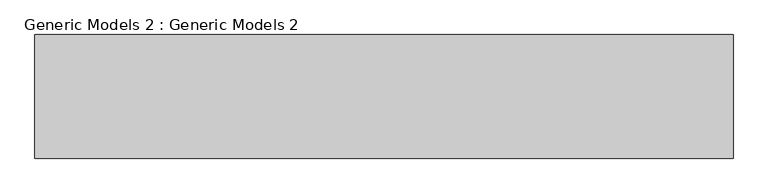
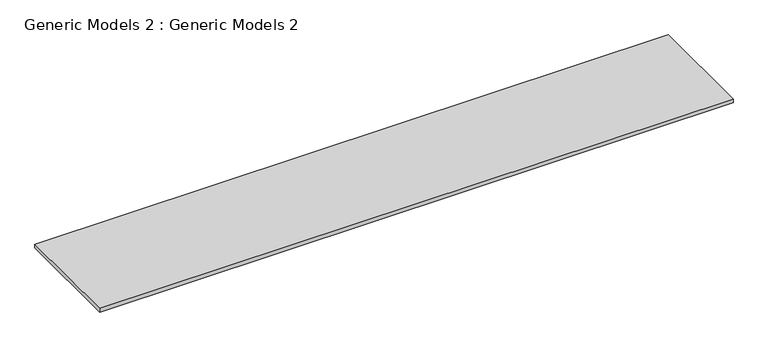
"""IFC4 building model written with IfcOpenShell, lengths in millimetres: proxy geometry, Generic Models 2 : Generic Models 2."""

from ifc_helpers import new_model, si_unit, frame, origin, place, context, project, spatial, polyline, outline, extrude, source, transform, mapped, element, save


def generic_models_2_generic_models_2_4f75562f(model_context):
    return source(origin(), model_context, "Body", "SweptSolid", [
        extrude(outline(polyline([(-13230.2331462, -12744.7202358), (12372.9668538, -12744.7202358), (12372.9668538, -17277.8412235), (-13230.2331462, -17277.8412235), (-13230.2331462, -12744.7202358)])), frame((0.0, 0.0, -152.4), z_axis=(0.0, 0.0, 1.0), x_axis=(1.0, 0.0, 0.0)), (0.0, 0.0, 1.0), 152.4),
    ])


if __name__ == "__main__":
    model = new_model("IFC4")
    model_context = context("Model", 3, world=origin())
    ifc_project = project(units=[si_unit("LENGTHUNIT", "METRE", prefix="MILLI")], contexts=[model_context])
    site = spatial("IfcSite", under=ifc_project)
    building = spatial("IfcBuilding", under=site)
    placement = place(None, origin())
    generic_models_2_generic_models_2_shape = generic_models_2_generic_models_2_4f75562f(model_context)
    element("IfcBuildingElementProxy", 1, Name="Generic Models 2 : Generic Models 2", ObjectType="Generic Models 2 : Generic Models 2", at=placement, inside=building, context=model_context, shape_type="MappedRepresentation", body=[
        mapped(generic_models_2_generic_models_2_shape, transform((0.0, 0.0, 0.0), x_axis=(1.0, 0.0, 0.0), y_axis=(0.0, 1.0, 0.0), z_axis=(0.0, 0.0, 1.0))),
    ])
    save(model, "model.ifc")
